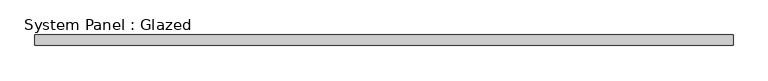
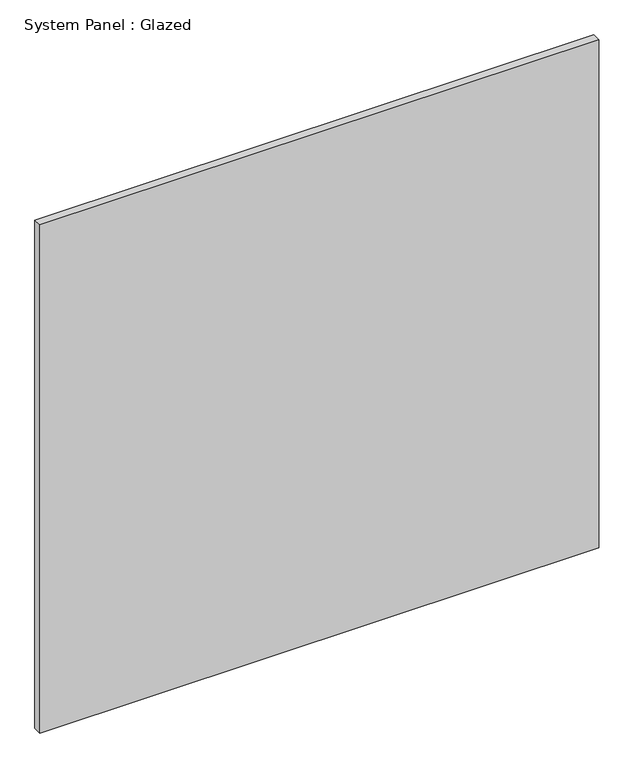
"""IFC4 building model written with IfcOpenShell, lengths in millimetres: plate geometry, System Panel : Glazed."""

from ifc_helpers import new_model, si_unit, origin, origin_with_axes, place, context, project, spatial, polyline, outline, extrude, source, transform, mapped, element, save


def system_panel_glazed_1654ed80(model_context):
    return source(origin(), model_context, "Body", "SweptSolid", [
        extrude(outline(polyline([(838.2, 19.05), (-838.2, 19.05), (-838.2, 44.45), (838.2, 44.45), (838.2, 19.05)])), origin_with_axes(), (0.0, 0.0, 1.0), 1611.4007577),
    ])


if __name__ == "__main__":
    model = new_model("IFC4")
    model_context = context("Model", 3, world=origin())
    ifc_project = project(units=[si_unit("LENGTHUNIT", "METRE", prefix="MILLI")], contexts=[model_context])
    site = spatial("IfcSite", under=ifc_project)
    building = spatial("IfcBuilding", under=site)
    placement = place(None, origin())
    system_panel_glazed_shape = system_panel_glazed_1654ed80(model_context)
    element("IfcPlate", 1, ObjectType="System Panel : Glazed", at=placement, inside=building, context=model_context, shape_type="MappedRepresentation", body=[
        mapped(system_panel_glazed_shape, transform((0.0, 0.0, 0.0), x_axis=(1.0, 0.0, 0.0), y_axis=(0.0, 1.0, 0.0), z_axis=(0.0, 0.0, 1.0))),
    ])
    save(model, "model.ifc")

# Revit data of these elements
# Type "System Panel : Glazed"
#   Construction Type Id = "GSP4R"
#   Analytic Construction = "1/8 in Pilkington single glazing"
#   Visual Light Transmittance = 0.9
#   Solar Heat Gain Coefficient = 0.86
#   Heat Transfer Coefficient (U) = 1.18115 BTU/(h·ft²·°F)
# Element 1 (IfcPlate, "System Panel : Glazed")
#   Materials on its faces: "Glass"
# Materials
#   "Glass": class "Glass", colour RGB 0 128 192, transparency 0.75, Description = "Soda Lime Glass", Cost = 0
